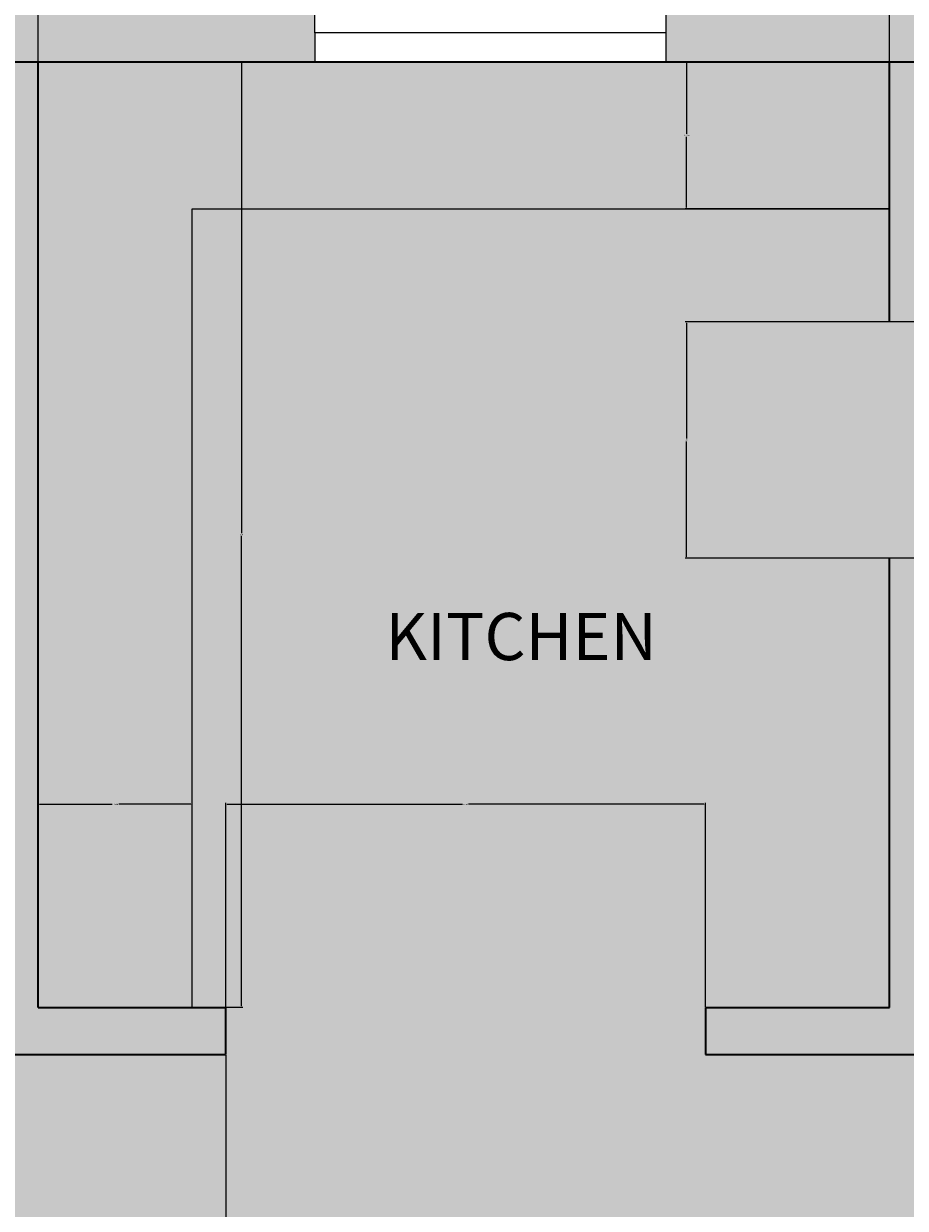
# Model space of a CAD drawing. Units: inches. Extents: x 3024 to 3952, y 1308 to 1863.
# Tile 25 of 29: x 3297 to 3409, y 1633 to 1783. Entities that reach past the tile are written whole.
import ezdxf

# ---------------------------------------------------------------- set-up
doc = ezdxf.new("R2010")
doc.units = ezdxf.units.IN
for name, color, linetype, lineweight in [('A-ANNO-DIMS', 2, 'Continuous', 18), ('A-AREA-IDEN', 7, 'Continuous', 18), ('A-DOOR', 4, 'Continuous', 18), ('A-FLOR-CASE', 8, 'Continuous', 18), ('A-FLOR-CASE-PATT', 47, 'Continuous', 13), ('A-FLOR-TILE-PATT', 7, 'Continuous', 13), ('A-GLAZ', 4, 'Continuous', 18), ('A-WALL', 7, 'Continuous', 35)]:
    doc.layers.add(name, color=color, linetype=linetype, lineweight=lineweight)
doc.layers.add('A-FLOR-PATT', color=254, linetype='Continuous', lineweight=13, true_color=0xfeeab9)
doc.layers.add('A-WALL-PATT', color=254, linetype='Continuous', lineweight=13, true_color=0xcecce6)
doc.styles.get("Standard").update_dxf_attribs({"font": 'arial.ttf'})
doc.dimstyles.get("Standard").update_dxf_attribs({"dimtxt": 0.18, "dimasz": 0.18, "dimexe": 0.18, "dimexo": 0.0625, "dimgap": 0.09, "dimtad": 0, "dimtih": 1, "dimtoh": 1, "dimdec": 4, "dimzin": 0, "dimdsep": 46, "dimtxsty": 'Standard', "dimcen": 0.09, "dimadec": 0, "dimazin": 0, "dimtfac": 1, "dimtdec": 4, "dimtofl": 0, "dimtmove": 0, "dimatfit": 3, "dimfxl": 1, "dimtolj": 1, "dimtzin": 0, "dimarcsym": 0})

# ---------------------------------------------------------------- blocks, each defined once
blk = doc.blocks.new('*U3')
for p, q in [((0, 0), (0, 6)), ((40, 0), (40, 6))]:
    blk.add_line(p, q)
blk.add_lwpolyline([(0, 0), (0, -40), (1.75, -40), (1.75, 0)], close=True)
blk.add_arc((0, 0), 40, 270, 0)
blk = doc.blocks.new('*D40')
at = {"layer": 'A-ANNO-DIMS', "color": 0, "lineweight": -2, "transparency": 16777216}
for p, q in [((3298.76, 1778.67), (3298.76, 1862.78)), ((3298.94, 1862.6), (3352.48, 1862.6)), ((3406.58, 1862.6), (3353.04, 1862.6)), ((3406.76, 1778.67), (3406.76, 1862.78))]:
    blk.add_line(p, q, dxfattribs=at)
at = {"layer": 'A-ANNO-DIMS', "color": 0, "transparency": 16777216}
for points in [[(3298.94, 1862.63), (3298.94, 1862.57), (3298.76, 1862.6)], [(3406.58, 1862.63), (3406.58, 1862.57), (3406.76, 1862.6)]]:
    blk.add_solid(points, dxfattribs=at)
at = {"layer": 'Defpoints', "color": 0, "transparency": 16777216}
for p in [(3406.76, 1862.6), (3298.76, 1778.61), (3406.76, 1778.61)]:
    blk.add_point(p, dxfattribs=at)
at = {"layer": 'A-ANNO-DIMS', "color": 0, "transparency": 16777216, "insert": (3352.76, 1862.6), "char_height": 0.18, "attachment_point": 5}
blk.add_mtext('\\A1;108', dxfattribs=at)
blk = doc.blocks.new('*D49')
at = {"layer": 'A-ANNO-DIMS', "color": 0, "lineweight": -2, "transparency": 16777216}
for p, q in [((3298.83, 1778.61), (3324.72, 1778.61)), ((3324.54, 1778.43), (3324.54, 1718.79)), ((3324.54, 1658.79), (3324.54, 1718.42)), ((3298.83, 1658.61), (3324.72, 1658.61))]:
    blk.add_line(p, q, dxfattribs=at)
at = {"layer": 'A-ANNO-DIMS', "color": 0, "transparency": 16777216}
for points in [[(3324.51, 1778.43), (3324.57, 1778.43), (3324.54, 1778.61)], [(3324.51, 1658.79), (3324.57, 1658.79), (3324.54, 1658.61)]]:
    blk.add_solid(points, dxfattribs=at)
at = {"layer": 'Defpoints', "color": 0, "transparency": 16777216}
for p in [(3298.76, 1778.61), (3298.76, 1658.61), (3324.54, 1658.61)]:
    blk.add_point(p, dxfattribs=at)
at = {"layer": 'A-ANNO-DIMS', "color": 0, "transparency": 16777216, "insert": (3324.54, 1718.61), "char_height": 0.18, "attachment_point": 5}
blk.add_mtext('\\A1;120', dxfattribs=at)
blk = doc.blocks.new('*D60')
at = {"layer": 'A-ANNO-DIMS', "color": 0, "lineweight": -2, "transparency": 16777216}
for p, q in [((3406.7, 1745.61), (3380.81, 1745.61)), ((3380.99, 1745.43), (3380.99, 1730.79)), ((3380.99, 1715.79), (3380.99, 1730.42)), ((3406.7, 1715.61), (3380.81, 1715.61))]:
    blk.add_line(p, q, dxfattribs=at)
at = {"layer": 'A-ANNO-DIMS', "color": 0, "transparency": 16777216}
for points in [[(3380.96, 1745.43), (3381.02, 1745.43), (3380.99, 1745.61)], [(3380.96, 1715.79), (3381.02, 1715.79), (3380.99, 1715.61)]]:
    blk.add_solid(points, dxfattribs=at)
at = {"layer": 'Defpoints', "color": 0, "transparency": 16777216}
for p in [(3380.99, 1745.61), (3406.76, 1745.61), (3406.76, 1715.61)]:
    blk.add_point(p, dxfattribs=at)
at = {"layer": 'A-ANNO-DIMS', "color": 0, "transparency": 16777216, "insert": (3380.99, 1730.61), "char_height": 0.18, "attachment_point": 5}
blk.add_mtext('\\A1;30', dxfattribs=at)
blk = doc.blocks.new('*D62')
at = {"layer": 'A-ANNO-DIMS', "color": 0, "lineweight": -2, "transparency": 16777216}
for p, q in [((3322.54, 1658.67), (3322.54, 1684.56)), ((3322.72, 1684.38), (3352.57, 1684.38)), ((3383.21, 1684.38), (3353.36, 1684.38)), ((3383.39, 1658.67), (3383.39, 1684.56))]:
    blk.add_line(p, q, dxfattribs=at)
at = {"layer": 'A-ANNO-DIMS', "color": 0, "transparency": 16777216}
for points in [[(3322.72, 1684.41), (3322.72, 1684.35), (3322.54, 1684.38)], [(3383.21, 1684.41), (3383.21, 1684.35), (3383.39, 1684.38)]]:
    blk.add_solid(points, dxfattribs=at)
at = {"layer": 'Defpoints', "color": 0, "transparency": 16777216}
for p in [(3383.39, 1684.38), (3322.54, 1658.61), (3383.39, 1658.61)]:
    blk.add_point(p, dxfattribs=at)
at = {"layer": 'A-ANNO-DIMS', "color": 0, "transparency": 16777216, "insert": (3352.96, 1684.38), "char_height": 0.18, "attachment_point": 5}
blk.add_mtext('\\A1;60.86', dxfattribs=at)
blk = doc.blocks.new('*D63')
at = {"layer": 'A-ANNO-DIMS', "color": 0, "lineweight": -2, "transparency": 16777216}
for p, q in [((3292.76, 1652.54), (3292.76, 1626.65)), ((3322.54, 1652.54), (3322.54, 1626.65)), ((3292.94, 1626.83), (3307.25, 1626.83)), ((3322.36, 1626.83), (3308.05, 1626.83))]:
    blk.add_line(p, q, dxfattribs=at)
at = {"layer": 'A-ANNO-DIMS', "color": 0, "transparency": 16777216}
for points in [[(3292.94, 1626.86), (3292.94, 1626.8), (3292.76, 1626.83)], [(3322.36, 1626.86), (3322.36, 1626.8), (3322.54, 1626.83)]]:
    blk.add_solid(points, dxfattribs=at)
at = {"layer": 'Defpoints', "color": 0, "transparency": 16777216}
for p in [(3292.76, 1652.61), (3322.54, 1652.61), (3292.76, 1626.83)]:
    blk.add_point(p, dxfattribs=at)
at = {"layer": 'A-ANNO-DIMS', "color": 0, "transparency": 16777216, "insert": (3307.65, 1626.83), "char_height": 0.18, "attachment_point": 5}
blk.add_mtext('\\A1;29.77', dxfattribs=at)
blk = doc.blocks.new('*D77')
at = {"layer": 'A-ANNO-DIMS', "color": 0, "lineweight": -2, "transparency": 16777216}
for p, q in [((3298.76, 1658.67), (3298.76, 1684.56)), ((3298.94, 1684.38), (3308.08, 1684.38)), ((3318.12, 1684.38), (3308.99, 1684.38)), ((3318.3, 1658.67), (3318.3, 1684.56))]:
    blk.add_line(p, q, dxfattribs=at)
at = {"layer": 'A-ANNO-DIMS', "color": 0, "transparency": 16777216}
for points in [[(3298.94, 1684.41), (3298.94, 1684.35), (3298.76, 1684.38)], [(3318.12, 1684.41), (3318.12, 1684.35), (3318.3, 1684.38)]]:
    blk.add_solid(points, dxfattribs=at)
at = {"layer": 'Defpoints', "color": 0, "transparency": 16777216}
for p in [(3318.3, 1684.38), (3298.76, 1658.61), (3318.3, 1658.61)]:
    blk.add_point(p, dxfattribs=at)
at = {"layer": 'A-ANNO-DIMS', "color": 0, "transparency": 16777216, "insert": (3308.53, 1684.38), "char_height": 0.18, "attachment_point": 5}
blk.add_mtext('\\A1;19.534', dxfattribs=at)
blk = doc.blocks.new('*D78')
at = {"layer": 'A-ANNO-DIMS', "color": 0, "lineweight": -2, "transparency": 16777216}
for p, q in [((3406.7, 1778.61), (3380.81, 1778.61)), ((3380.99, 1778.43), (3380.99, 1769.46)), ((3380.99, 1760.13), (3380.99, 1769.1)), ((3406.7, 1759.95), (3380.81, 1759.95))]:
    blk.add_line(p, q, dxfattribs=at)
at = {"layer": 'A-ANNO-DIMS', "color": 0, "transparency": 16777216}
for points in [[(3380.96, 1778.43), (3381.02, 1778.43), (3380.99, 1778.61)], [(3380.96, 1760.13), (3381.02, 1760.13), (3380.99, 1759.95)]]:
    blk.add_solid(points, dxfattribs=at)
at = {"layer": 'Defpoints', "color": 0, "transparency": 16777216}
for p in [(3380.99, 1778.61), (3406.76, 1778.61), (3406.76, 1759.95)]:
    blk.add_point(p, dxfattribs=at)
at = {"layer": 'A-ANNO-DIMS', "color": 0, "transparency": 16777216, "insert": (3380.99, 1769.28), "char_height": 0.18, "attachment_point": 5}
blk.add_mtext('\\A1;18.655', dxfattribs=at)

msp = doc.modelspace()

# ---------------------------------------------------------------- hatches: boundary and pattern name
at = {"layer": 'A-FLOR-CASE-PATT'}
h = msp.add_hatch(color=256, dxfattribs=at)
h.dxf.hatch_style = 1
h.paths.add_polyline_path([(3318.2981, 1759.9514), (3406.764, 1759.9514), (3406.764, 1778.6064), (3298.764, 1778.6064), (3298.764, 1658.6064), (3318.2981, 1658.6064)])
at = {"layer": 'A-FLOR-PATT', "transparency": 33554528}
h = msp.add_hatch(color=256, dxfattribs=at)
h.dxf.hatch_style = 1
h.paths.add_polyline_path([(3460.764, 1688.6064), (3412.764, 1688.6064), (3412.764, 1694.6064), (3460.764, 1694.6064), (3460.764, 1778.6064), (3406.764, 1778.6064), (3406.764, 1759.9514), (3318.2981, 1759.9514), (3318.2981, 1658.6064), (3322.5356, 1658.6064), (3322.5356, 1652.6064), (3292.764, 1652.6064), (3292.764, 1778.6064), (3106.764, 1778.6064), (3106.764, 1628.6064), (3172.764, 1628.6064), (3172.764, 1532.6064), (3166.764, 1532.6064), (3166.764, 1628.6064), (3106.764, 1628.6064), (3106.764, 1356.8452), (3202.812, 1356.8452), (3202.812, 1354.2534), (3202.812, 1353.8388), (3202.812, 1351.1212), (3202.812, 1347.8452), (3277.764, 1347.8452), (3277.764, 1353.8452), (3277.764, 1356.8452), (3277.764, 1442.6064), (3460.764, 1442.6064)])
h.paths.add_polyline_path([(3216.238, 1527.2064), (3216.238, 1491.2064), (3214.663, 1491.2064), (3214.663, 1491.2409, -0.39662236), (3180.243, 1526.6064), (3163.0285, 1526.6064), (3163.0285, 1531.1064), (3161.716, 1531.1064), (3161.716, 1561.1064), (3163.0285, 1561.1064), (3163.0285, 1531.1064), (3163.0285, 1526.6064), (3180.243, 1526.6064, 0.39662236), (3214.663, 1491.2409), (3214.663, 1527.2064)], flags=16)
h.paths.add_polyline_path([(3227.364, 1649.8972), (3191.364, 1649.8972), (3191.364, 1651.4722), (3227.364, 1651.4722)], flags=16)
h.paths.add_polyline_path([(3323.1172, 1606.7362), (3323.8545, 1606.8514), (3323.8545, 1594.8241), (3323.1172, 1594.9393)], flags=16)
h.paths.add_polyline_path([(3324.2232, 1606.909), (3330.1216, 1607.8307), (3330.1216, 1614.1093), (3339.3495, 1614.1093), (3340.2711, 1620.0078), (3352.4136, 1620.0078), (3353.3353, 1614.1093), (3359.9941, 1614.1093), (3360.9157, 1620.0078), (3373.0582, 1620.0078), (3373.9799, 1614.1093), (3383.2077, 1614.1093), (3383.2077, 1607.8307), (3389.1062, 1606.909), (3389.1062, 1594.7665), (3383.2077, 1593.8449), (3383.2077, 1587.5663), (3373.9799, 1587.5663), (3373.0583, 1581.6678), (3360.9157, 1581.6678), (3359.9941, 1587.5663), (3353.3353, 1587.5663), (3352.4136, 1581.6678), (3340.2711, 1581.6678), (3339.3495, 1587.5663), (3330.1216, 1587.5663), (3330.1216, 1593.8449), (3324.2232, 1594.7665)], flags=16)
h.paths.add_polyline_path([(3236.1584, 1693.1064), (3236.1584, 1723.1064), (3237.4709, 1723.1064), (3237.4709, 1693.1064)], flags=16)
h.paths.add_polyline_path([(3373.2158, 1600.6847), (3373.7965, 1600.7303), (3374.3268, 1600.7874), (3374.8132, 1600.8531), (3375.2621, 1600.9247), (3375.6801, 1600.9991), (3376.0736, 1601.0735), (3376.6855, 1601.19), (3377.366, 1601.3023), (3378.0667, 1601.3814), (3378.8026, 1601.4123), (3379.5865, 1601.3839), (3380.4537, 1601.2948), (3381.301, 1601.1717), (3382.0317, 1601.0433), (3382.4398, 1600.9607), (3382.6252, 1600.9201), (3382.919, 1600.8507), (3382.9044, 1600.8531), (3382.842, 1600.8678), (3382.7541, 1600.8896), (3382.6252, 1600.9201), (3382.4398, 1600.9607), (3382.1868, 1601.0119), (3381.8738, 1601.0711), (3381.5125, 1601.1346), (3381.1149, 1601.1988), (3380.6928, 1601.2601), (3380.2581, 1601.3149), (3379.8226, 1601.3597), (3379.3984, 1601.3908), (3378.9944, 1601.4054), (3378.6092, 1601.4042), (3378.2384, 1601.3886), (3377.8777, 1601.36), (3377.5227, 1601.32), (3377.1691, 1601.2698), (3376.8127, 1601.211), (3376.4491, 1601.145), (3376.0736, 1601.0735), (3375.4177, 1600.9494), (3374.5542, 1600.8119), (3373.5044, 1600.6988)], flags=0)
h.paths.add_polyline_path([(3380.0253, 1596.7351), (3380.499, 1596.6659), (3380.9706, 1596.6119), (3381.4375, 1596.5791), (3381.8971, 1596.5736), (3382.5886, 1596.6167), (3382.7848, 1596.6692), (3382.1465, 1596.5706), (3381.236, 1596.5815), (3380.3199, 1596.6865)], flags=0)
h.paths.add_polyline_path([(3369.6414, 1603.9617), (3370.1589, 1604.0021), (3370.6218, 1604.0539), (3371.0335, 1604.1173), (3371.3978, 1604.1921), (3371.7181, 1604.2785), (3371.9984, 1604.3761), (3372.2441, 1604.483), (3372.4611, 1604.5972), (3372.655, 1604.7163), (3372.8317, 1604.8384), (3372.9968, 1604.9611), (3373.3703, 1605.2455), (3373.8426, 1605.5328), (3374.4624, 1605.7539), (3375.1058, 1605.8302), (3375.7221, 1605.8261), (3376.4109, 1605.76), (3377.1534, 1605.6376), (3377.8945, 1605.473), (3378.1382, 1605.409), (3377.7394, 1605.5074), (3377.3509, 1605.5937), (3376.9704, 1605.6677), (3376.5999, 1605.7288), (3376.2417, 1605.7762), (3375.8979, 1605.8092), (3375.5707, 1605.8271), (3375.2621, 1605.8291), (3374.9745, 1605.8146), (3374.7092, 1605.7832), (3374.4647, 1605.7359), (3374.239, 1605.6742), (3374.0298, 1605.5996), (3373.835, 1605.5134), (3373.6525, 1605.4171), (3373.4801, 1605.3123), (3373.3156, 1605.2002), (3373.1562, 1605.0825), (3372.7603, 1604.781), (3372.236, 1604.4588), (3371.5738, 1604.2283), (3370.8493, 1604.0794), (3369.9262, 1603.976)], flags=0)
h.paths.add_polyline_path([(3366.7533, 1606.5832), (3367.1713, 1606.5519), (3367.5378, 1606.5374), (3367.8568, 1606.5394), (3368.1325, 1606.5573), (3368.3694, 1606.5903), (3368.5717, 1606.6377), (3368.7438, 1606.6988), (3368.89, 1606.7728), (3369.0146, 1606.8591), (3369.121, 1606.9568), (3369.2094, 1607.0646), (3369.2792, 1607.181), (3369.3295, 1607.3046), (3369.3596, 1607.4339), (3369.3688, 1607.5676), (3369.3565, 1607.7042), (3369.3218, 1607.8422), (3369.2649, 1607.9804), (3369.1893, 1608.1187), (3369.0993, 1608.2569), (3368.9992, 1608.3952), (3368.8934, 1608.5334), (3368.7861, 1608.6717), (3368.6817, 1608.8099), (3368.4212, 1609.1804), (3368.2685, 1609.7106), (3368.4883, 1610.1814), (3369.0537, 1610.4604), (3369.6717, 1610.5097), (3370.2812, 1610.3612), (3370.4805, 1610.2968), (3370.1882, 1610.3839), (3369.9284, 1610.4472), (3369.6905, 1610.4842), (3369.4662, 1610.4933), (3369.2555, 1610.4765), (3369.0608, 1610.4367), (3368.884, 1610.3767), (3368.7274, 1610.2994), (3368.5931, 1610.2077), (3368.4833, 1610.1045), (3368.4002, 1609.9927), (3368.3451, 1609.8747), (3368.3166, 1609.7517), (3368.3127, 1609.6244), (3368.331, 1609.4935), (3368.3696, 1609.3597), (3368.4261, 1609.2237), (3368.4985, 1609.0863), (3368.5845, 1608.9482), (3368.6817, 1608.8099), (3368.7861, 1608.6717), (3368.8934, 1608.5334), (3368.9992, 1608.3952), (3369.0993, 1608.2569), (3369.3398, 1607.8876), (3369.3941, 1607.2896), (3368.9774, 1606.7817), (3368.3928, 1606.5742), (3367.7162, 1606.5303), (3367.0044, 1606.5585)], flags=0)
h.paths.add_polyline_path([(3362.1859, 1610.2589), (3362.5478, 1610.2845), (3362.8348, 1610.3275), (3363.0585, 1610.3863), (3363.2303, 1610.4595), (3363.3619, 1610.5457), (3363.463, 1610.6432), (3363.5376, 1610.7502), (3363.5876, 1610.8643), (3363.6153, 1610.9834), (3363.6229, 1611.1055), (3363.6125, 1611.2283), (3363.5861, 1611.3496), (3363.5462, 1611.4673), (3363.4949, 1611.5797), (3363.4358, 1611.6871), (3363.3723, 1611.7902), (3363.3081, 1611.8897), (3363.2468, 1611.9863), (3363.192, 1612.0808), (3363.0258, 1612.4261), (3363.3371, 1612.8672), (3363.9008, 1612.9782), (3364.4822, 1612.9641), (3365.1098, 1612.9074), (3365.328, 1612.8805), (3364.9615, 1612.9208), (3364.6426, 1612.9496), (3364.3668, 1612.9669), (3364.1299, 1612.9726), (3363.9276, 1612.9669), (3363.7555, 1612.9496), (3363.6093, 1612.9208), (3363.4848, 1612.8805), (3363.3782, 1612.8289), (3363.2889, 1612.7672), (3363.2169, 1612.6969), (3363.1622, 1612.6193), (3363.1247, 1612.5361), (3363.1046, 1612.4484), (3363.1017, 1612.358), (3363.1161, 1612.266), (3363.1472, 1612.1738), (3363.192, 1612.0808), (3363.2468, 1611.9863), (3363.3081, 1611.8897), (3363.3723, 1611.7902), (3363.4358, 1611.6871), (3363.6363, 1611.323), (3363.5979, 1610.7003), (3363.0863, 1610.3651), (3362.3983, 1610.2622)], flags=0)
h.paths.add_polyline_path([(3352.356, 1581.2991), (3352.2408, 1580.5618), (3340.4439, 1580.5618), (3340.3287, 1581.2991)], flags=16)
h.paths.add_polyline_path([(3340.4439, 1621.1137), (3352.2408, 1621.1137), (3352.356, 1620.3764), (3340.3287, 1620.3764)], flags=16)
h.paths.add_polyline_path([(3278.4282, 1504.7424), (3290.3831, 1504.7424), (3290.3831, 1502.7499), (3291.0473, 1502.7499), (3291.0473, 1494.7799), (3290.3831, 1494.7799), (3290.3831, 1494.1158), (3291.0473, 1494.1158), (3291.0473, 1486.1458), (3290.3831, 1486.1458), (3290.3831, 1484.1533), (3291.0473, 1484.1533), (3291.0473, 1483.4892, -0.09090909), (3291.0473, 1468.8776), (3291.0473, 1468.2135), (3290.3831, 1468.2135), (3290.3831, 1464.8926), (3278.4282, 1464.8926), (3278.4282, 1472.8626), (3277.764, 1473.5268), (3277.764, 1478.84), (3278.4282, 1479.5042)], flags=16)
h.paths.add_polyline_path([(3278.7603, 1504.4103), (3290.051, 1504.4103), (3290.051, 1465.2247), (3278.7603, 1465.2247)], flags=0)
h.paths.add_polyline_path([(3123.904, 1600.7821), (3117.9039, 1602.7821), (3117.9039, 1599.7821), (3119.4039, 1599.7821), (3119.4039, 1596.7821), (3118.4039, 1596.7821), (3118.4039, 1598.7821), (3117.9039, 1598.7821), (3117.9039, 1596.2821), (3109.9039, 1596.2821), (3109.9039, 1617.2821), (3117.9039, 1617.2821), (3117.9039, 1610.7821), (3123.9038, 1612.7821, -0.70257121), (3137.9039, 1606.7822, -0.70256205)], flags=16)
h.paths.add_polyline_path([(3123.9039, 1602.7822), (3123.9039, 1610.7822, -0.73453329), (3136.9039, 1606.7822, -0.73452973)], flags=0)
h.paths.add_polyline_path([(3177.972, 1689.6473), (3109.2405, 1689.6473), (3109.2405, 1741.1959), (3177.972, 1741.1959)], flags=16)
h.paths.add_polyline_path([(3373.0006, 1581.2991), (3372.8854, 1580.5618), (3361.0885, 1580.5618), (3360.9733, 1581.2991)], flags=16)
h.paths.add_polyline_path([(3361.0885, 1621.1137), (3372.8854, 1621.1137), (3373.0006, 1620.3764), (3360.9733, 1620.3764)], flags=16)
h.paths.add_polyline_path([(3116.9039, 1598.2821, -0.41421356), (3116.1539, 1597.2821), (3111.9039, 1597.2821, -0.41421356), (3110.9039, 1598.0321), (3110.9039, 1615.2821, -0.41421356), (3111.6539, 1616.2821), (3115.9039, 1616.2821, -0.41421356), (3116.9039, 1615.5321)], flags=0)
h.paths.add_polyline_path([(3121.6122, 1728.1369), (3121.6122, 1696.5205), (3110.2715, 1696.5205), (3110.2715, 1714.3906), (3121.6122, 1714.3906), (3121.6122, 1716.4526), (3110.2715, 1716.4526), (3110.2715, 1734.3228), (3123.3304, 1734.3228), (3123.3304, 1729.8552), (3134.6711, 1741.1959), (3134.6711, 1728.1369)], flags=0)
h.paths.add_polyline_path([(3389.4748, 1606.8514), (3390.2122, 1606.7362), (3390.2122, 1594.9393), (3389.4748, 1594.8241)], flags=16)
h.paths.add_polyline_path([(3257.6842, 1762.8281), (3259.6842, 1768.8281), (3256.6842, 1768.8281), (3256.6842, 1767.3281), (3253.6842, 1767.3281), (3253.6842, 1768.3281), (3255.6842, 1768.3281), (3255.6842, 1768.8281), (3253.1842, 1768.8281), (3253.1842, 1776.8281), (3274.1842, 1776.8281), (3274.1842, 1768.8281), (3267.6842, 1768.8281), (3269.6842, 1762.8282, -0.70257121), (3263.6843, 1748.8282, -0.70256205)], flags=16)
h.paths.add_polyline_path([(3259.6842, 1762.8281), (3267.6843, 1762.8281, -0.73453329), (3263.6842, 1749.8282, -0.73452973)], flags=0)
h.paths.add_polyline_path([(3411.264, 1715.6064), (3411.264, 1716.9189), (3441.264, 1716.9189), (3441.264, 1715.6064)], flags=16)
h.paths.add_polyline_path([(3178.3806, 1449.1876), (3178.3806, 1397.639), (3109.6491, 1397.639), (3109.6491, 1449.1876)], flags=16)
h.paths.add_polyline_path([(3397.1501, 1541.7146), (3419.6183, 1541.7146), (3419.6183, 1496.7783), (3397.1501, 1496.7783)], flags=16)
h.paths.add_polyline_path([(3254.1842, 1770.5781), (3254.1842, 1774.8281, -0.41421356), (3254.9342, 1775.8281), (3272.1842, 1775.8281, -0.41421356), (3273.1842, 1775.0781), (3273.1842, 1770.8281, -0.41421356), (3272.4342, 1769.8281), (3255.1842, 1769.8281, -0.41421356)], flags=0)
h.paths.add_polyline_path([(3403.672, 1500.7601), (3403.6016, 1500.3997), (3403.5328, 1500.0441), (3403.4662, 1499.6867), (3403.4027, 1499.3226), (3403.3464, 1498.9532), (3403.3025, 1498.5811), (3403.2759, 1498.2091), (3403.2714, 1497.8401), (3403.3064, 1497.2813), (3403.3491, 1497.1219), (3403.2689, 1497.6395), (3403.2778, 1498.3719), (3403.3635, 1499.0984), (3403.4889, 1499.8168), (3403.6016, 1500.3997), (3403.672, 1500.7601), (3403.744, 1501.1315), (3403.817, 1501.5205), (3403.891, 1501.9336), (3403.9656, 1502.3769), (3404.0404, 1502.8572), (3404.115, 1503.3786), (3404.2264, 1504.2311), (3404.2571, 1504.5223), (3404.1552, 1503.6598), (3404.0063, 1502.6193), (3403.8604, 1501.7518), (3403.744, 1501.1315)], flags=0)
h.paths.add_polyline_path([(3406.5868, 1505.0416), (3406.6121, 1504.5236), (3406.6492, 1504.0526), (3406.6956, 1503.624), (3406.7491, 1503.2333), (3406.8072, 1502.8759), (3406.8676, 1502.5473), (3406.9281, 1502.243), (3407.0268, 1501.7597), (3407.1416, 1501.1368), (3407.2087, 1500.3904), (3407.1804, 1499.6703), (3407.1078, 1498.9956), (3407.0074, 1498.3199), (3406.8809, 1497.6059), (3406.7403, 1496.9627), (3406.7418, 1496.9824), (3406.7491, 1497.0249), (3406.8229, 1497.3409), (3406.8364, 1497.4025), (3406.878, 1497.6078), (3406.9261, 1497.8614), (3406.9777, 1498.1526), (3407.0298, 1498.4712), (3407.0797, 1498.8068), (3407.1243, 1499.149), (3407.1607, 1499.4874), (3407.1859, 1499.8115), (3407.1978, 1500.1137), (3407.1969, 1500.3962), (3407.1841, 1500.6642), (3407.1609, 1500.9225), (3407.1284, 1501.1761), (3407.0876, 1501.43), (3407.0398, 1501.6891), (3406.9862, 1501.9585), (3406.8832, 1502.4628), (3406.7712, 1503.0713), (3406.6657, 1503.8424), (3406.5924, 1504.7735)], flags=0)
h.paths.add_polyline_path([(3409.2517, 1507.8962), (3409.2752, 1507.4282), (3409.3079, 1507.0076), (3409.3501, 1506.6314), (3409.4015, 1506.2969), (3409.4624, 1506.0009), (3409.5326, 1505.7406), (3409.6119, 1505.5128), (3409.6988, 1505.3131), (3409.7915, 1505.1368), (3409.8883, 1504.9792), (3409.9875, 1504.8356), (3410.0872, 1504.7015), (3410.1859, 1504.572), (3410.4508, 1504.2132), (3410.7205, 1503.6035), (3410.8059, 1502.8824), (3410.7619, 1502.0875), (3410.6122, 1501.2299), (3410.4402, 1500.6169), (3410.2538, 1500.0031), (3410.0536, 1499.3219), (3409.9909, 1499.0812), (3410.1761, 1499.7472), (3410.3596, 1500.3513), (3410.4512, 1500.6561), (3410.5312, 1500.9412), (3410.6013, 1501.226), (3410.6614, 1501.512), (3410.7111, 1501.7964), (3410.7496, 1502.0763), (3410.7764, 1502.3489), (3410.7909, 1502.6114), (3410.7926, 1502.8608), (3410.7808, 1503.0944), (3410.7553, 1503.31), (3410.7169, 1503.5087), (3410.6667, 1503.6921), (3410.6061, 1503.8621), (3410.5361, 1504.0203), (3410.4578, 1504.1686), (3410.3726, 1504.3088), (3410.2815, 1504.4424), (3410.1859, 1504.572), (3410.0872, 1504.7015), (3409.859, 1505.0083), (3409.5943, 1505.5117), (3409.4266, 1506.1336), (3409.324, 1506.8011), (3409.2586, 1507.6407)], flags=0)
h.paths.add_polyline_path([(3411.4914, 1510.5878), (3411.4432, 1510.1586), (3411.4054, 1509.775), (3411.38, 1509.4354), (3411.3681, 1509.1376), (3411.3698, 1508.8784), (3411.3843, 1508.6542), (3411.4112, 1508.4618), (3411.4497, 1508.2974), (3411.4994, 1508.1575), (3411.5595, 1508.0388), (3411.6296, 1507.9375), (3411.7097, 1507.851), (3411.802, 1507.7792), (3411.9096, 1507.7225), (3412.0353, 1507.6817), (3412.1821, 1507.6572), (3412.3528, 1507.6496), (3412.5505, 1507.6597), (3412.778, 1507.6879), (3413.0364, 1507.7341), (3413.3194, 1507.7955), (3413.6188, 1507.8687), (3413.9264, 1507.95), (3414.234, 1508.036), (3414.5333, 1508.1232), (3414.8163, 1508.208), (3415.0747, 1508.287), (3415.3023, 1508.3569), (3415.5007, 1508.4158), (3415.6733, 1508.4617), (3416.1158, 1508.5538), (3416.512, 1508.2591), (3416.716, 1507.6581), (3416.61, 1507.0003), (3416.3052, 1506.3411), (3415.8928, 1505.618), (3415.7339, 1505.3633), (3415.9914, 1505.791), (3416.201, 1506.1583), (3416.3666, 1506.4739), (3416.4925, 1506.7462), (3416.5828, 1506.9838), (3416.6413, 1507.1949), (3416.6725, 1507.3883), (3416.6799, 1507.5705), (3416.6662, 1507.7417), (3416.6339, 1507.9), (3416.5851, 1508.0436), (3416.5223, 1508.1709), (3416.4478, 1508.28), (3416.3639, 1508.3692), (3416.273, 1508.4368), (3416.1765, 1508.4815), (3416.0718, 1508.5047), (3415.9553, 1508.5079), (3415.8237, 1508.493), (3415.6733, 1508.4617), (3415.5007, 1508.4158), (3415.3327, 1508.3659), (3414.6495, 1508.157), (3414.0606, 1507.9855), (3413.4456, 1507.8229), (3412.8838, 1507.701), (3412.5505, 1507.6597), (3412.0748, 1507.6354), (3411.595, 1507.8883), (3411.398, 1508.4429), (3411.3624, 1508.9927), (3411.3854, 1509.5711), (3411.4578, 1510.3071)], flags=0)
h.paths.add_polyline_path([(3135.0797, 1449.1876), (3135.0797, 1436.1286), (3122.0208, 1436.1286), (3122.0208, 1404.5122), (3110.6801, 1404.5122), (3110.6801, 1422.3823), (3122.0208, 1422.3823), (3122.0208, 1424.4443), (3110.6801, 1424.4443), (3110.6801, 1442.3145), (3123.739, 1442.3145), (3123.739, 1437.8469)], flags=0)
h.paths.add_polyline_path([(3416.4944, 1514.2949), (3416.4837, 1513.8511), (3416.4893, 1513.4867), (3416.5102, 1513.1926), (3416.5451, 1512.9593), (3416.5929, 1512.7775), (3416.6524, 1512.6379), (3416.7224, 1512.531), (3416.8017, 1512.4488), (3416.8886, 1512.3882), (3416.9813, 1512.3476), (3417.0781, 1512.3251), (3417.1773, 1512.3189), (3417.277, 1512.3274), (3417.3757, 1512.3488), (3417.4713, 1512.3813), (3417.5627, 1512.4229), (3417.65, 1512.471), (3417.7338, 1512.5225), (3417.8146, 1512.5747), (3417.8931, 1512.6245), (3417.9699, 1512.6691), (3418.2968, 1512.8265), (3418.6505, 1512.4645), (3418.7037, 1511.9342), (3418.6693, 1511.3839), (3418.6076, 1510.8228), (3418.5777, 1510.5927), (3418.6197, 1510.9333), (3418.6525, 1511.2311), (3418.6759, 1511.4903), (3418.6899, 1511.7144), (3418.6946, 1511.9069), (3418.6899, 1512.0713), (3418.6759, 1512.2112), (3418.6525, 1512.33), (3418.6197, 1512.4311), (3418.5778, 1512.5177), (3418.5276, 1512.5903), (3418.4705, 1512.6488), (3418.4075, 1512.6933), (3418.3399, 1512.7237), (3418.2686, 1512.7401), (3418.1951, 1512.7424), (3418.1204, 1512.7307), (3418.0455, 1512.7055), (3417.9792, 1512.6736), (3417.65, 1512.471), (3417.5627, 1512.4229), (3417.4713, 1512.3813), (3417.3757, 1512.3488), (3417.277, 1512.3274), (3416.878, 1512.2936), (3416.5757, 1512.7549), (3416.492, 1513.3145), (3416.4808, 1514.0384)], flags=0)
h.paths.add_polyline_path([(3392.8223, 1481.9454), (3396.7707, 1481.9454), (3396.7707, 1480.9201), (3428.3585, 1480.9201), (3428.3585, 1481.9454), (3432.3069, 1481.9454), (3432.3069, 1464.8354, -0.26666697), (3392.8223, 1464.8354)], flags=16)
h.paths.add_polyline_path([(3431.203, 1547.5428), (3450.8613, 1547.5428, -0.19047621), (3450.8614, 1484.031), (3431.203, 1484.031), (3431.203, 1488.5675), (3432.3809, 1488.5675), (3432.3809, 1543.0062), (3431.203, 1543.0062)], flags=16)
h.paths.add_polyline_path([(3451.9233, 1524.86, -0.04962821), (3451.9233, 1506.7138), (3446.7921, 1506.7138), (3446.7921, 1524.86)], flags=0)
h.paths.add_polyline_path([(3460.764, 1436.6064), (3277.764, 1436.6064), (3277.764, 1356.8452), (3277.764, 1353.8452), (3460.764, 1353.8452)], flags=17)
h.paths.add_polyline_path([(3121.3033, 1577.378), (3153.693, 1577.378), (3153.693, 1586.6752), (3121.3033, 1586.6752)], flags=24)
h.paths.add_polyline_path([(3164.1457, 1464.1276), (3210.4801, 1464.1276), (3210.4801, 1473.4247), (3164.1457, 1473.4247)], flags=24)
h.paths.add_polyline_path([(3343.1909, 1505.8863), (3373.7236, 1505.8863), (3373.7236, 1515.1773), (3343.1909, 1515.1773)], flags=24)
h.paths.add_polyline_path([(3337.6353, 1564.2926), (3370.0189, 1564.2926), (3370.0189, 1573.5836), (3337.6353, 1573.5836)], flags=24)
h.paths.add_polyline_path([(3419.204, 1753.8578), (3453.3997, 1753.8578), (3453.3997, 1762.9956), (3419.204, 1762.9956)], flags=24)
h.paths.add_polyline_path([(3341.2523, 1701.0246), (3381.0761, 1701.0246), (3381.0761, 1710.3156), (3341.2523, 1710.3156)], flags=24)
h.paths.add_polyline_path([(3245.8895, 1726.2997), (3278.2793, 1726.2997), (3278.2793, 1735.5968), (3245.8895, 1735.5968)], flags=24)
h.paths.add_polyline_path([(3128.8045, 1668.6736), (3175.1389, 1668.6736), (3175.1389, 1677.9707), (3128.8045, 1677.9707)], flags=24)
h.paths.add_polyline_path([(3345.9997, 1396.0062), (3389.09, 1396.0062), (3389.09, 1405.3033), (3345.9997, 1405.3033)], flags=24)
at = {"layer": 'A-FLOR-TILE-PATT', "transparency": 33554569}
h = msp.add_hatch(dxfattribs=at)
h.set_pattern_fill('ANGLE', color=256, scale=2)
h.set_pattern_definition([(0, (0, 0), (0, 13.97), [10.16, -3.81]), (90, (0, 0), (-13.97, 9e-16), [10.16, -3.81])])
h.paths.add_polyline_path([(3292.764, 1778.6064), (3232.764, 1778.6064), (3232.764, 1694.6064), (3236.1584, 1694.6064), (3236.1584, 1723.1064), (3237.4709, 1723.1064), (3237.4709, 1723.0777, -0.38700389), (3266.1209, 1694.6064), (3292.764, 1694.6064)])
h.paths.add_polyline_path([(3263.6843, 1748.8282, -0.70256205), (3257.6842, 1762.8281), (3259.6842, 1768.8281), (3256.6842, 1768.8281), (3256.6842, 1767.3281), (3253.6842, 1767.3281), (3253.6842, 1768.3281), (3255.6842, 1768.3281), (3255.6842, 1768.8281), (3253.1842, 1768.8281), (3253.1842, 1776.8281), (3274.1842, 1776.8281), (3274.1842, 1768.8281), (3267.6842, 1768.8281), (3269.6842, 1762.8282, -0.70257121)], flags=16)
h.paths.add_polyline_path([(3263.6842, 1749.8282, -0.73452973), (3259.6842, 1762.8281), (3267.6843, 1762.8281, -0.73453329)], flags=0)
h.paths.add_polyline_path([(3255.1842, 1769.8281, -0.41421356), (3254.1842, 1770.5781), (3254.1842, 1774.8281, -0.41421356), (3254.9342, 1775.8281), (3272.1842, 1775.8281, -0.41421356), (3273.1842, 1775.0781), (3273.1842, 1770.8281, -0.41421356), (3272.4342, 1769.8281)], flags=0)
h.paths.add_polyline_path([(3460.764, 1436.6064), (3277.764, 1436.6064), (3277.764, 1356.8452), (3277.764, 1353.8452), (3460.764, 1353.8452)])
h.paths.add_polyline_path([(3166.764, 1628.6064), (3106.764, 1628.6064), (3106.764, 1532.6064), (3133.066, 1532.6064, -0.38700389), (3161.716, 1561.0777), (3161.716, 1561.1064), (3163.0285, 1561.1064), (3163.0285, 1532.6064), (3166.764, 1532.6064)])
h.paths.add_polyline_path([(3123.904, 1600.7821), (3117.9039, 1602.7821), (3117.9039, 1599.7821), (3119.4039, 1599.7821), (3119.4039, 1596.7821), (3118.4039, 1596.7821), (3118.4039, 1598.7821), (3117.9039, 1598.7821), (3117.9039, 1596.2821), (3109.9039, 1596.2821), (3109.9039, 1617.2821), (3117.9039, 1617.2821), (3117.9039, 1610.7821), (3123.9038, 1612.7821, -0.70257121), (3137.9039, 1606.7822, -0.70256205)], flags=16)
h.paths.add_polyline_path([(3123.9039, 1602.7822), (3123.9039, 1610.7822, -0.73453329), (3136.9039, 1606.7822, -0.73452973)], flags=0)
h.paths.add_polyline_path([(3116.1539, 1597.2821), (3111.9039, 1597.2821, -0.41421356), (3110.9039, 1598.0321), (3110.9039, 1615.2821, -0.41421356), (3111.6539, 1616.2821), (3115.9039, 1616.2821, -0.41421356), (3116.9039, 1615.5321), (3116.9039, 1598.2821, -0.41421356)], flags=0)
h.paths.add_polyline_path([(3245.8895, 1726.2997), (3278.2793, 1726.2997), (3278.2793, 1735.5968), (3245.8895, 1735.5968)], flags=24)
h.paths.add_polyline_path([(3345.9997, 1396.0062), (3389.09, 1396.0062), (3389.09, 1405.3033), (3345.9997, 1405.3033)], flags=24)
h.paths.add_polyline_path([(3121.3033, 1577.378), (3153.693, 1577.378), (3153.693, 1586.6752), (3121.3033, 1586.6752)], flags=24)
at = {"layer": 'A-WALL-PATT'}
h = msp.add_hatch(color=256, dxfattribs=at)
h.dxf.hatch_style = 1
h.paths.add_polyline_path([(3106.764, 1778.6064), (3140.5977, 1778.6064), (3140.5977, 1781.8824), (3140.5977, 1784.6), (3140.5977, 1787.6064), (3097.764, 1787.6064), (3097.764, 1590.213), (3101.04, 1590.213), (3103.7576, 1590.213), (3106.764, 1590.213)])
h.paths.add_polyline_path([(3253.5314, 1781.8824), (3253.5314, 1784.6), (3253.5314, 1787.6064), (3194.6826, 1787.6064), (3194.6826, 1785.0146), (3194.6826, 1784.6), (3194.6826, 1781.8824), (3194.6826, 1778.6064), (3253.5314, 1778.6064)])
h.paths.add_polyline_path([(3333.856, 1782.2838), (3333.856, 1784.7474), (3333.856, 1787.6064), (3272.0523, 1787.6064), (3272.0523, 1785.0146), (3272.0523, 1784.6), (3272.0523, 1781.8824), (3272.0523, 1778.6064), (3333.856, 1778.6064)])
h.paths.add_polyline_path([(3428.8344, 1784.6), (3428.8344, 1787.6064), (3378.3947, 1787.6064), (3378.3947, 1784.7474), (3378.3947, 1782.2838), (3378.3947, 1778.6064), (3428.8344, 1778.6064), (3428.8344, 1781.8824)], flags=17)
h.paths.add_polyline_path([(3469.764, 1787.6064), (3451.9386, 1787.6064), (3451.9386, 1785.0146), (3451.9386, 1784.6), (3451.9386, 1781.8824), (3451.9386, 1778.6064), (3460.764, 1778.6064), (3460.764, 1353.8452), (3277.764, 1353.8452), (3277.764, 1347.8452), (3469.764, 1347.8452), (3469.764, 1353.8452)])
h.paths.add_polyline_path([(3106.764, 1571.6922), (3104.1722, 1571.6922), (3103.7576, 1571.6922), (3101.04, 1571.6922), (3097.764, 1571.6922), (3097.764, 1347.8452), (3148.7271, 1347.8452), (3148.7271, 1351.1212), (3148.7271, 1353.8388), (3148.7271, 1356.8452), (3106.764, 1356.8452)])
h.paths.add_polyline_path([(3277.764, 1532.6064), (3262.7605, 1532.6064), (3262.7605, 1582.9359), (3256.7605, 1582.9359), (3256.7605, 1532.6064), (3244.2116, 1532.6064), (3216.238, 1532.6064), (3216.238, 1527.2064), (3216.238, 1526.6064), (3271.764, 1526.6064), (3271.764, 1356.8452), (3202.812, 1356.8452), (3202.812, 1354.2534), (3202.812, 1353.8388), (3202.812, 1351.1212), (3202.812, 1347.8452), (3277.764, 1347.8452), (3277.764, 1353.8452), (3277.764, 1356.8452)])
h.paths.add_polyline_path([(3180.238, 1532.6064), (3163.0285, 1532.6064), (3163.0285, 1531.1064), (3163.0285, 1526.6064), (3180.243, 1526.6064, -0.00416688), (3180.238, 1527.2064)])
h.paths.add_polyline_path([(3133.0285, 1531.1064, -0.01250587), (3133.066, 1532.6064), (3106.764, 1532.6064), (3106.764, 1526.6064), (3133.0285, 1526.6064)], flags=17)
h.paths.add_polyline_path([(3172.764, 1628.6064), (3166.764, 1628.6064), (3166.764, 1532.6064), (3172.764, 1532.6064)])
h.paths.add_polyline_path([(3232.764, 1649.8972), (3227.364, 1649.8972), (3226.764, 1649.8972), (3226.764, 1634.6064), (3106.764, 1634.6064), (3106.764, 1628.6064), (3232.764, 1628.6064)])
h = msp.add_hatch(color=256, dxfattribs=at)
h.dxf.hatch_style = 1
h.paths.add_polyline_path([(3232.764, 1778.6064), (3226.764, 1778.6064), (3226.764, 1685.8922, -0.00416688), (3227.364, 1685.8972), (3232.764, 1685.8972)])
h.paths.add_polyline_path([(3298.764, 1778.6064), (3292.764, 1778.6064), (3292.764, 1652.6064), (3322.5356, 1652.6064), (3322.5356, 1658.6064), (3298.764, 1658.6064)])
h.paths.add_polyline_path([(3412.764, 1715.6064), (3411.264, 1715.6064), (3406.764, 1715.6064), (3406.764, 1658.6064), (3383.3911, 1658.6064), (3383.3911, 1652.6064), (3412.764, 1652.6064)])
h.paths.add_polyline_path([(3412.764, 1778.6064), (3406.764, 1778.6064), (3406.764, 1745.6064), (3411.264, 1745.6064, -0.01250587), (3412.764, 1745.5689)])

# ---------------------------------------------------------------- linework, layer by layer
at = {"layer": 'A-FLOR-CASE'}
for p, q in [((3318.2981, 1658.6064), (3318.2981, 1759.9514)), ((3318.2981, 1759.9514), (3406.764, 1759.9514))]:
    msp.add_line(p, q, dxfattribs=at)
at = {"layer": 'A-GLAZ'}
for p, q in [((3333.856, 1782.2838), (3333.856, 1778.6064)), ((3378.3947, 1782.2838), (3378.3947, 1778.6064))]:
    msp.add_line(p, q, dxfattribs=at)
msp.add_lwpolyline([(3333.856, 1784.7474), (3378.3947, 1784.7474), (3378.3947, 1782.2838), (3333.856, 1782.2838)], close=True, dxfattribs=at)
at = {"layer": 'A-WALL'}
for p, q in [((3106.764, 1778.6064), (3460.764, 1778.6064)), ((3298.764, 1658.6064), (3298.764, 1778.6064)), ((3406.764, 1745.6064), (3406.764, 1778.6064)), ((3406.764, 1658.6064), (3406.764, 1715.6064)), ((3298.764, 1658.6064), (3322.5356, 1658.6064)), ((3322.5356, 1658.6064), (3322.5356, 1652.6064)), ((3383.3911, 1658.6064), (3383.3911, 1652.6064)), ((3383.3911, 1658.6064), (3406.764, 1658.6064)), ((3292.764, 1652.6064), (3322.5356, 1652.6064)), ((3383.3911, 1652.6064), (3412.764, 1652.6064))]:
    msp.add_line(p, q, dxfattribs=at)

# ---------------------------------------------------------------- block references
at = {"layer": 'A-DOOR', "xscale": 0.75, "yscale": 0.75, "zscale": 0.75, "rotation": 90}
msp.add_blockref('*U3', (3411.264, 1715.6064), dxfattribs=at)

# ---------------------------------------------------------------- texts
at = {"layer": 'A-AREA-IDEN'}
msp.add_text('KITCHEN', height=5.98971, dxfattribs=at).set_placement((3342.8008, 1702.6752))

# ---------------------------------------------------------------- dimensions: what is measured, and where the dimension line sits
at = {"layer": 'A-ANNO-DIMS'}
for base, p1, p2, override, picture, middle in [((3406.764, 1862.6031), (3298.764, 1778.6064), (3406.764, 1778.6064), {"dimdec": 0, "dimlfac": 1, "dimrnd": 0, "dimzin": 0, "dimdsep": 46, "dimlunit": 2}, '*D40', (3352.764, 1862.6031)), ((3318.2981, 1684.3814), (3298.764, 1658.6064), (3318.2981, 1658.6064), {"dimdec": 3, "dimlfac": 1, "dimrnd": 0, "dimzin": 0, "dimdsep": 46, "dimlunit": 2}, '*D77', (3308.5311, 1684.3814)), ((3383.3911, 1684.3814), (3322.5356, 1658.6064), (3383.3911, 1658.6064), {"dimdec": 2, "dimlfac": 1, "dimrnd": 0, "dimzin": 0, "dimdsep": 46, "dimlunit": 2}, '*D62', (3352.9634, 1684.3814))]:
    dim = msp.add_linear_dim(base=base, p1=p1, p2=p2, dimstyle='Standard', override=override, dxfattribs=at)
    dim.commit()
    dim.dimension.update_dxf_attribs({"geometry": picture, "text_midpoint": middle})
for base, p1, p2, angle, override, picture, middle in [((3324.539, 1658.6064), (3298.764, 1778.6064), (3298.764, 1658.6064), 270, {"dimdec": 0, "dimlfac": 1, "dimrnd": 0, "dimzin": 0, "dimdsep": 46, "dimlunit": 2}, '*D49', (3324.539, 1718.6064)), ((3380.989, 1778.6064), (3406.764, 1759.9514), (3406.764, 1778.6064), 90, {"dimdec": 3, "dimlfac": 1, "dimrnd": 0, "dimzin": 0, "dimdsep": 46, "dimlunit": 2}, '*D78', (3380.989, 1769.2789)), ((3380.989, 1745.6064), (3406.764, 1715.6064), (3406.764, 1745.6064), 90, {"dimdec": 0, "dimlfac": 1, "dimrnd": 0, "dimzin": 0, "dimdsep": 46, "dimlunit": 2}, '*D60', (3380.989, 1730.6064)), ((3292.764, 1626.8314), (3322.5356, 1652.6064), (3292.764, 1652.6064), 180, {"dimdec": 2, "dimlfac": 1, "dimrnd": 0, "dimzin": 0, "dimdsep": 46, "dimlunit": 2}, '*D63', (3307.6498, 1626.8314))]:
    dim = msp.add_linear_dim(base=base, p1=p1, p2=p2, angle=angle, dimstyle='Standard', override=override, dxfattribs=at)
    dim.commit()
    dim.dimension.update_dxf_attribs({"geometry": picture, "text_midpoint": middle})

doc.saveas('drawing.dxf')
